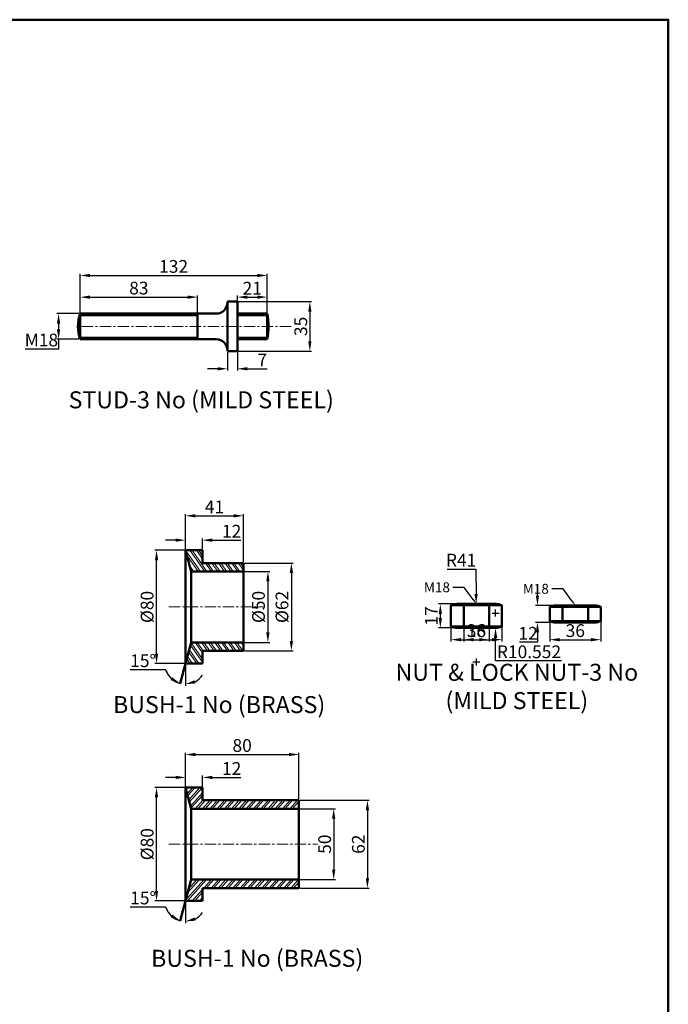
# Model space of a CAD drawing. Units: millimetres. Extents: x -98 to 907, y -783 to 313.
# Tile 3 of 3: x 449 to 907, y -383 to 313. Entities that reach past the tile are written whole.
import ezdxf
from ezdxf import colors
from ezdxf.entities.mleader import LeaderData, LeaderLine
from ezdxf.math import Vec2, Vec3

# ---------------------------------------------------------------- set-up
doc = ezdxf.new("R2010")
doc.units = ezdxf.units.MM
doc.header["$LTSCALE"] = 0.5
doc.linetypes.add('CENTER', pattern=[50.8, 31.75, -6.35, 6.35, -6.35])
for name, color, linetype, lineweight in [('M-CNTR', 1, 'CENTER', 18), ('M-DIMS', 2, 'Continuous', 25), ('M-HATC', 8, 'Continuous', 18), ('M-OUTL', 7, 'Continuous', 50), ('M-TEXT', 3, 'Continuous', 25)]:
    doc.layers.add(name, color=color, linetype=linetype, lineweight=lineweight)
doc.styles.get("Standard").update_dxf_attribs({"font": 'arial.ttf'})
doc.dimstyles.new('ISO-25', dxfattribs={"dimtxt": 9, "dimasz": 7, "dimexe": 1.25, "dimexo": 0.625, "dimtad": 1, "dimtoh": 1, "dimtxsty": 'Standard', "dimcen": 2.5, "dimadec": 0, "dimazin": 0, "dimtfac": 1, "dimtofl": 0, "dimtmove": 0, "dimatfit": 3, "dimfxl": 1, "dimarcsym": 0})

# ---------------------------------------------------------------- blocks, each defined once
blk = doc.blocks.new('*D15')
at = {"layer": 'Defpoints', "color": 0, "ltscale": 0.5, "transparency": 16777216}
for p in [(623.45, 132.18), (491.45, 105.21), (623.45, 105.21)]:
    blk.add_point(p, dxfattribs=at)
at = {"layer": 'M-DIMS', "color": 0, "lineweight": -2, "ltscale": 0.5, "transparency": 16777216}
for p, q in [((491.45, 105.84), (491.45, 133.43)), ((498.45, 132.18), (616.45, 132.18)), ((623.45, 105.84), (623.45, 133.43))]:
    blk.add_line(p, q, dxfattribs=at)
at = {"layer": 'M-DIMS', "color": 0, "ltscale": 0.5, "transparency": 16777216}
for points in [[(498.45, 133.35), (498.45, 131.02), (491.45, 132.18)], [(616.45, 133.35), (616.45, 131.02), (623.45, 132.18)]]:
    blk.add_solid(points, dxfattribs=at)
at = {"layer": 'M-DIMS', "color": 0, "ltscale": 0.5, "transparency": 16777216, "insert": (557.45, 137.41), "char_height": 9, "attachment_point": 5}
blk.add_mtext('132', dxfattribs=at)
blk = doc.blocks.new('*D16')
at = {"layer": 'Defpoints', "color": 0, "ltscale": 0.5, "transparency": 16777216}
for p in [(491.45, 111.42), (574.45, 116.88), (574.45, 104.21)]:
    blk.add_point(p, dxfattribs=at)
at = {"layer": 'M-DIMS', "color": 0, "lineweight": -2, "ltscale": 0.5, "transparency": 16777216}
for p, q in [((491.45, 112.04), (491.45, 118.13)), ((498.45, 116.88), (567.45, 116.88)), ((574.45, 104.84), (574.45, 118.13))]:
    blk.add_line(p, q, dxfattribs=at)
at = {"layer": 'M-DIMS', "color": 0, "ltscale": 0.5, "transparency": 16777216}
for points in [[(498.45, 118.04), (498.45, 115.71), (491.45, 116.88)], [(567.45, 118.04), (567.45, 115.71), (574.45, 116.88)]]:
    blk.add_solid(points, dxfattribs=at)
at = {"layer": 'M-DIMS', "color": 0, "ltscale": 0.5, "transparency": 16777216, "insert": (532.95, 122.1), "char_height": 9, "attachment_point": 5}
blk.add_mtext('83', dxfattribs=at)
blk = doc.blocks.new('*D17')
at = {"layer": 'Defpoints', "color": 0, "ltscale": 0.5, "transparency": 16777216}
for p in [(491.45, 105.21), (476.29, 87.21), (491.45, 87.21)]:
    blk.add_point(p, dxfattribs=at)
at = {"layer": 'M-DIMS', "color": 0, "lineweight": -2, "ltscale": 0.5, "transparency": 16777216}
for p, q in [((490.83, 105.21), (475.04, 105.21)), ((476.29, 98.21), (476.29, 94.21)), ((490.83, 87.21), (475.04, 87.21)), ((476.29, 87.21), (476.29, 80.21)), ((476.29, 80.21), (452.69, 80.21))]:
    blk.add_line(p, q, dxfattribs=at)
at = {"layer": 'M-DIMS', "color": 0, "ltscale": 0.5, "transparency": 16777216}
for points in [[(475.13, 98.21), (477.46, 98.21), (476.29, 105.21)], [(475.13, 94.21), (477.46, 94.21), (476.29, 87.21)]]:
    blk.add_solid(points, dxfattribs=at)
at = {"layer": 'M-DIMS', "color": 0, "ltscale": 0.5, "transparency": 16777216, "insert": (464.18, 85.43), "char_height": 9, "attachment_point": 5}
blk.add_mtext('M18', dxfattribs=at)
blk = doc.blocks.new('*D18')
at = {"layer": 'Defpoints', "color": 0, "ltscale": 0.5, "transparency": 16777216}
for p in [(595.45, 78.71), (602.45, 78.71), (602.45, 66.27)]:
    blk.add_point(p, dxfattribs=at)
at = {"layer": 'M-DIMS', "color": 0, "lineweight": -2, "ltscale": 0.5, "transparency": 16777216}
for p, q in [((595.45, 78.09), (595.45, 65.02)), ((602.45, 78.09), (602.45, 65.02)), ((588.45, 66.27), (581.45, 66.27)), ((609.45, 66.27), (623.53, 66.27))]:
    blk.add_line(p, q, dxfattribs=at)
at = {"layer": 'M-DIMS', "color": 0, "ltscale": 0.5, "transparency": 16777216}
for points in [[(588.45, 67.43), (588.45, 65.1), (595.45, 66.27)], [(609.45, 67.43), (609.45, 65.1), (602.45, 66.27)]]:
    blk.add_solid(points, dxfattribs=at)
at = {"layer": 'M-DIMS', "color": 0, "ltscale": 0.5, "transparency": 16777216, "insert": (619.99, 71.39), "char_height": 9, "attachment_point": 5}
blk.add_mtext('7', dxfattribs=at)
blk = doc.blocks.new('*D19')
at = {"layer": 'Defpoints', "color": 0, "ltscale": 0.5, "transparency": 16777216}
for p in [(602.45, 113.71), (623.45, 116.88), (623.45, 113.71)]:
    blk.add_point(p, dxfattribs=at)
at = {"layer": 'M-DIMS', "color": 0, "lineweight": -2, "ltscale": 0.5, "transparency": 16777216}
for p, q in [((602.45, 114.34), (602.45, 118.13)), ((609.45, 116.88), (616.45, 116.88)), ((623.45, 114.34), (623.45, 118.13))]:
    blk.add_line(p, q, dxfattribs=at)
at = {"layer": 'M-DIMS', "color": 0, "ltscale": 0.5, "transparency": 16777216}
for points in [[(609.45, 118.04), (609.45, 115.71), (602.45, 116.88)], [(616.45, 118.04), (616.45, 115.71), (623.45, 116.88)]]:
    blk.add_solid(points, dxfattribs=at)
at = {"layer": 'M-DIMS', "color": 0, "ltscale": 0.5, "transparency": 16777216, "insert": (612.95, 122.02), "char_height": 9, "attachment_point": 5}
blk.add_mtext('21', dxfattribs=at)
blk = doc.blocks.new('*D20')
at = {"layer": 'Defpoints', "color": 0, "ltscale": 0.5, "transparency": 16777216}
for p in [(602.45, 113.71), (602.45, 78.71), (653.62, 78.71)]:
    blk.add_point(p, dxfattribs=at)
at = {"layer": 'M-DIMS', "color": 0, "lineweight": -2, "ltscale": 0.5, "transparency": 16777216}
for p, q in [((603.08, 113.71), (654.87, 113.71)), ((653.62, 106.71), (653.62, 85.71)), ((603.08, 78.71), (654.87, 78.71))]:
    blk.add_line(p, q, dxfattribs=at)
at = {"layer": 'M-DIMS', "color": 0, "ltscale": 0.5, "transparency": 16777216}
for points in [[(652.45, 106.71), (654.78, 106.71), (653.62, 113.71)], [(652.45, 85.71), (654.78, 85.71), (653.62, 78.71)]]:
    blk.add_solid(points, dxfattribs=at)
at = {"layer": 'M-DIMS', "color": 0, "ltscale": 0.5, "transparency": 16777216, "insert": (648.39, 96.21), "char_height": 9, "attachment_point": 5, "rotation": 90}
blk.add_mtext('35', dxfattribs=at)
blk = doc.blocks.new('*D21')
at = {"layer": 'Defpoints', "color": 0, "ltscale": 0.5, "transparency": 16777216}
for p in [(577.83, -54.77), (565.83, -61.94), (577.83, -61.94)]:
    blk.add_point(p, dxfattribs=at)
at = {"layer": 'M-DIMS', "color": 0, "lineweight": -2, "ltscale": 0.5, "transparency": 16777216}
for p, q in [((558.83, -54.77), (551.83, -54.77)), ((565.83, -61.31), (565.83, -53.52)), ((577.83, -61.31), (577.83, -53.52)), ((584.83, -54.77), (605.03, -54.77))]:
    blk.add_line(p, q, dxfattribs=at)
at = {"layer": 'M-DIMS', "color": 0, "ltscale": 0.5, "transparency": 16777216}
for points in [[(558.83, -53.6), (558.83, -55.94), (565.83, -54.77)], [(584.83, -53.6), (584.83, -55.94), (577.83, -54.77)]]:
    blk.add_solid(points, dxfattribs=at)
at = {"layer": 'M-DIMS', "color": 0, "ltscale": 0.5, "transparency": 16777216, "insert": (598.43, -49.63), "char_height": 9, "attachment_point": 5}
blk.add_mtext('12', dxfattribs=at)
blk = doc.blocks.new('*D22')
at = {"layer": 'Defpoints', "color": 0, "ltscale": 0.5, "transparency": 16777216}
for p in [(606.83, -37.58), (565.83, -61.94), (606.83, -70.94)]:
    blk.add_point(p, dxfattribs=at)
at = {"layer": 'M-DIMS', "color": 0, "lineweight": -2, "ltscale": 0.5, "transparency": 16777216}
for p, q in [((565.83, -61.31), (565.83, -36.33)), ((572.83, -37.58), (599.83, -37.58)), ((606.83, -70.31), (606.83, -36.33))]:
    blk.add_line(p, q, dxfattribs=at)
at = {"layer": 'M-DIMS', "color": 0, "ltscale": 0.5, "transparency": 16777216}
for points in [[(572.83, -36.41), (572.83, -38.74), (565.83, -37.58)], [(599.83, -36.41), (599.83, -38.74), (606.83, -37.58)]]:
    blk.add_solid(points, dxfattribs=at)
at = {"layer": 'M-DIMS', "color": 0, "ltscale": 0.5, "transparency": 16777216, "insert": (586.33, -32.43), "char_height": 9, "attachment_point": 5}
blk.add_mtext('41', dxfattribs=at)
blk = doc.blocks.new('*D23')
at = {"layer": 'Defpoints', "color": 0, "ltscale": 0.5, "transparency": 16777216}
for p in [(606.83, -70.94), (606.83, -132.94), (640.59, -132.94)]:
    blk.add_point(p, dxfattribs=at)
at = {"layer": 'M-DIMS', "color": 0, "lineweight": -2, "ltscale": 0.5, "transparency": 16777216}
for p, q in [((607.45, -70.94), (641.84, -70.94)), ((640.59, -77.94), (640.59, -125.94)), ((607.45, -132.94), (641.84, -132.94))]:
    blk.add_line(p, q, dxfattribs=at)
at = {"layer": 'M-DIMS', "color": 0, "ltscale": 0.5, "transparency": 16777216}
for points in [[(639.42, -77.94), (641.76, -77.94), (640.59, -70.94)], [(639.42, -125.94), (641.76, -125.94), (640.59, -132.94)]]:
    blk.add_solid(points, dxfattribs=at)
at = {"layer": 'M-DIMS', "color": 0, "ltscale": 0.5, "transparency": 16777216, "insert": (635.12, -101.94), "char_height": 9, "attachment_point": 5, "rotation": 90}
blk.add_mtext('%%C62', dxfattribs=at)
blk = doc.blocks.new('*D24')
at = {"layer": 'Defpoints', "color": 0, "ltscale": 0.5, "transparency": 16777216}
for p in [(606.83, -76.94), (606.83, -126.94), (624.02, -126.94)]:
    blk.add_point(p, dxfattribs=at)
at = {"layer": 'M-DIMS', "color": 0, "lineweight": -2, "ltscale": 0.5, "transparency": 16777216}
for p, q in [((607.45, -76.94), (625.27, -76.94)), ((624.02, -83.94), (624.02, -119.94)), ((607.45, -126.94), (625.27, -126.94))]:
    blk.add_line(p, q, dxfattribs=at)
at = {"layer": 'M-DIMS', "color": 0, "ltscale": 0.5, "transparency": 16777216}
for points in [[(622.85, -83.94), (625.18, -83.94), (624.02, -76.94)], [(622.85, -119.94), (625.18, -119.94), (624.02, -126.94)]]:
    blk.add_solid(points, dxfattribs=at)
at = {"layer": 'M-DIMS', "color": 0, "ltscale": 0.5, "transparency": 16777216, "insert": (618.54, -101.94), "char_height": 9, "attachment_point": 5, "rotation": 90}
blk.add_mtext('%%C50', dxfattribs=at)
blk = doc.blocks.new('*D25')
at = {"layer": 'Defpoints', "color": 0, "ltscale": 0.5, "transparency": 16777216}
for p in [(545.42, -61.94), (565.83, -61.94), (565.83, -141.94)]:
    blk.add_point(p, dxfattribs=at)
at = {"layer": 'M-DIMS', "color": 0, "lineweight": -2, "ltscale": 0.5, "transparency": 16777216}
for p, q in [((565.2, -61.94), (544.17, -61.94)), ((545.42, -134.94), (545.42, -68.94)), ((565.2, -141.94), (544.17, -141.94))]:
    blk.add_line(p, q, dxfattribs=at)
at = {"layer": 'M-DIMS', "color": 0, "ltscale": 0.5, "transparency": 16777216}
for points in [[(544.26, -68.94), (546.59, -68.94), (545.42, -61.94)], [(544.26, -134.94), (546.59, -134.94), (545.42, -141.94)]]:
    blk.add_solid(points, dxfattribs=at)
at = {"layer": 'M-DIMS', "color": 0, "ltscale": 0.5, "transparency": 16777216, "insert": (539.95, -101.94), "char_height": 9, "attachment_point": 5, "rotation": 90}
blk.add_mtext('%%C80', dxfattribs=at)
blk = doc.blocks.new('*D26')
at = {"layer": 'Defpoints', "color": 0, "ltscale": 0.5, "transparency": 16777216}
for p in [(565.83, -101.94), (569.85, -126.94), (565.83, -141.94), (562.06, -156), (564.56, -156.44)]:
    blk.add_point(p, dxfattribs=at)
at = {"layer": 'M-DIMS', "color": 0, "lineweight": -2, "ltscale": 0.5, "transparency": 16777216}
for p, q in [((565.83, -142.56), (565.83, -157.74)), ((551.95, -146.31), (526.89, -146.31))]:
    blk.add_line(p, q, dxfattribs=at)
for start, end in [(197.5003, 255), (199.33739, 227.16869), (297.83131, 325.66261)]:
    blk.add_arc((565.83, -141.94), 14.55, start, end, dxfattribs=at)
at = {"layer": 'M-DIMS', "color": 0, "ltscale": 0.5, "transparency": 16777216}
for points in [[(556.5, -151.59), (555.37, -153.63), (562.06, -156)], [(572.9, -155.94), (572.34, -153.68), (565.83, -156.49)]]:
    blk.add_solid(points, dxfattribs=at)
at = {"layer": 'M-DIMS', "color": 0, "ltscale": 0.5, "transparency": 16777216, "insert": (535.92, -141.09), "char_height": 9, "attachment_point": 5}
blk.add_mtext('15°', dxfattribs=at)
blk = doc.blocks.new('*D29')
at = {"layer": 'Defpoints', "color": 0, "ltscale": 0.5, "transparency": 16777216}
for p in [(577.83, -222.33), (565.83, -229.5), (577.83, -229.5)]:
    blk.add_point(p, dxfattribs=at)
at = {"layer": 'M-DIMS', "color": 0, "lineweight": -2, "ltscale": 0.5, "transparency": 16777216}
for p, q in [((558.83, -222.33), (551.83, -222.33)), ((565.83, -228.88), (565.83, -221.08)), ((577.83, -228.88), (577.83, -221.08)), ((584.83, -222.33), (605.03, -222.33))]:
    blk.add_line(p, q, dxfattribs=at)
at = {"layer": 'M-DIMS', "color": 0, "ltscale": 0.5, "transparency": 16777216}
for points in [[(558.83, -221.17), (558.83, -223.5), (565.83, -222.33)], [(584.83, -221.17), (584.83, -223.5), (577.83, -222.33)]]:
    blk.add_solid(points, dxfattribs=at)
at = {"layer": 'M-DIMS', "color": 0, "ltscale": 0.5, "transparency": 16777216, "insert": (598.43, -217.19), "char_height": 9, "attachment_point": 5}
blk.add_mtext('12', dxfattribs=at)
blk = doc.blocks.new('*D27')
at = {"layer": 'Defpoints', "color": 0, "ltscale": 0.5, "transparency": 16777216}
for p in [(545.42, -229.5), (565.83, -229.5), (565.83, -309.5)]:
    blk.add_point(p, dxfattribs=at)
at = {"layer": 'M-DIMS', "color": 0, "lineweight": -2, "ltscale": 0.5, "transparency": 16777216}
for p, q in [((565.2, -229.5), (544.17, -229.5)), ((545.42, -302.5), (545.42, -236.5)), ((565.2, -309.5), (544.17, -309.5))]:
    blk.add_line(p, q, dxfattribs=at)
at = {"layer": 'M-DIMS', "color": 0, "ltscale": 0.5, "transparency": 16777216}
for points in [[(544.26, -236.5), (546.59, -236.5), (545.42, -229.5)], [(544.26, -302.5), (546.59, -302.5), (545.42, -309.5)]]:
    blk.add_solid(points, dxfattribs=at)
at = {"layer": 'M-DIMS', "color": 0, "ltscale": 0.5, "transparency": 16777216, "insert": (539.95, -269.5), "char_height": 9, "attachment_point": 5, "rotation": 90}
blk.add_mtext('%%C80', dxfattribs=at)
blk = doc.blocks.new('*D28')
at = {"layer": 'Defpoints', "color": 0, "ltscale": 0.5, "transparency": 16777216}
for p in [(565.83, -269.5), (569.85, -294.5), (565.83, -309.5), (562.06, -323.56), (564.56, -324)]:
    blk.add_point(p, dxfattribs=at)
at = {"layer": 'M-DIMS', "color": 0, "lineweight": -2, "ltscale": 0.5, "transparency": 16777216}
for p, q in [((565.83, -310.13), (565.83, -325.31)), ((551.95, -313.88), (526.89, -313.88))]:
    blk.add_line(p, q, dxfattribs=at)
for start, end in [(197.5003, 255), (199.33739, 227.16869), (297.83131, 325.66261)]:
    blk.add_arc((565.83, -309.5), 14.55, start, end, dxfattribs=at)
at = {"layer": 'M-DIMS', "color": 0, "ltscale": 0.5, "transparency": 16777216}
for points in [[(556.5, -319.15), (555.37, -321.2), (562.06, -323.56)], [(572.9, -323.51), (572.34, -321.24), (565.83, -324.06)]]:
    blk.add_solid(points, dxfattribs=at)
at = {"layer": 'M-DIMS', "color": 0, "ltscale": 0.5, "transparency": 16777216, "insert": (535.92, -308.66), "char_height": 9, "attachment_point": 5}
blk.add_mtext('15°', dxfattribs=at)
blk = doc.blocks.new('*D30')
at = {"layer": 'Defpoints', "color": 0, "ltscale": 0.5, "transparency": 16777216}
for p in [(645.83, -244.5), (645.83, -294.5), (670.45, -294.5)]:
    blk.add_point(p, dxfattribs=at)
at = {"layer": 'M-DIMS', "color": 0, "lineweight": -2, "ltscale": 0.5, "transparency": 16777216}
for p, q in [((646.45, -244.5), (671.7, -244.5)), ((670.45, -251.5), (670.45, -287.5)), ((646.45, -294.5), (671.7, -294.5))]:
    blk.add_line(p, q, dxfattribs=at)
at = {"layer": 'M-DIMS', "color": 0, "ltscale": 0.5, "transparency": 16777216}
for points in [[(669.29, -251.5), (671.62, -251.5), (670.45, -244.5)], [(669.29, -287.5), (671.62, -287.5), (670.45, -294.5)]]:
    blk.add_solid(points, dxfattribs=at)
at = {"layer": 'M-DIMS', "color": 0, "ltscale": 0.5, "transparency": 16777216, "insert": (665.23, -269.5), "char_height": 9, "attachment_point": 5, "rotation": 90}
blk.add_mtext('50', dxfattribs=at)
blk = doc.blocks.new('*D31')
at = {"layer": 'Defpoints', "color": 0, "ltscale": 0.5, "transparency": 16777216}
for p in [(645.83, -238.5), (645.83, -300.5), (694.26, -300.5)]:
    blk.add_point(p, dxfattribs=at)
at = {"layer": 'M-DIMS', "color": 0, "lineweight": -2, "ltscale": 0.5, "transparency": 16777216}
for p, q in [((646.45, -238.5), (695.51, -238.5)), ((694.26, -245.5), (694.26, -293.5)), ((646.45, -300.5), (695.51, -300.5))]:
    blk.add_line(p, q, dxfattribs=at)
at = {"layer": 'M-DIMS', "color": 0, "ltscale": 0.5, "transparency": 16777216}
for points in [[(693.09, -245.5), (695.42, -245.5), (694.26, -238.5)], [(693.09, -293.5), (695.42, -293.5), (694.26, -300.5)]]:
    blk.add_solid(points, dxfattribs=at)
at = {"layer": 'M-DIMS', "color": 0, "ltscale": 0.5, "transparency": 16777216, "insert": (689.04, -269.5), "char_height": 9, "attachment_point": 5, "rotation": 90}
blk.add_mtext('62', dxfattribs=at)
blk = doc.blocks.new('*D32')
at = {"layer": 'Defpoints', "color": 0, "ltscale": 0.5, "transparency": 16777216}
for p in [(645.83, -206.17), (565.83, -229.5), (645.83, -238.5)]:
    blk.add_point(p, dxfattribs=at)
at = {"layer": 'M-DIMS', "color": 0, "lineweight": -2, "ltscale": 0.5, "transparency": 16777216}
for p, q in [((565.83, -228.88), (565.83, -204.92)), ((572.83, -206.17), (638.83, -206.17)), ((645.83, -237.88), (645.83, -204.92))]:
    blk.add_line(p, q, dxfattribs=at)
at = {"layer": 'M-DIMS', "color": 0, "ltscale": 0.5, "transparency": 16777216}
for points in [[(572.83, -205.01), (572.83, -207.34), (565.83, -206.17)], [(638.83, -205.01), (638.83, -207.34), (645.83, -206.17)]]:
    blk.add_solid(points, dxfattribs=at)
at = {"layer": 'M-DIMS', "color": 0, "ltscale": 0.5, "transparency": 16777216, "insert": (605.83, -200.95), "char_height": 9, "attachment_point": 5}
blk.add_mtext('80', dxfattribs=at)
blk = doc.blocks.new('*D33')
at = {"layer": 'Defpoints', "color": 0, "ltscale": 0.5, "transparency": 16777216}
for p in [(762.2, -99.8), (745.71, -116.8), (762.2, -116.8)]:
    blk.add_point(p, dxfattribs=at)
at = {"layer": 'M-DIMS', "color": 0, "lineweight": -2, "ltscale": 0.5, "transparency": 16777216}
for p, q in [((761.57, -99.8), (744.46, -99.8)), ((745.71, -106.8), (745.71, -109.8)), ((761.57, -116.8), (744.46, -116.8))]:
    blk.add_line(p, q, dxfattribs=at)
at = {"layer": 'M-DIMS', "color": 0, "ltscale": 0.5, "transparency": 16777216}
for points in [[(744.54, -106.8), (746.87, -106.8), (745.71, -99.8)], [(744.54, -109.8), (746.87, -109.8), (745.71, -116.8)]]:
    blk.add_solid(points, dxfattribs=at)
at = {"layer": 'M-DIMS', "color": 0, "ltscale": 0.5, "transparency": 16777216, "insert": (740.56, -108.3), "char_height": 9, "attachment_point": 5, "rotation": 90}
blk.add_mtext('17', dxfattribs=at)
blk = doc.blocks.new('*D34')
at = {"layer": 'Defpoints', "color": 0, "ltscale": 0.5, "transparency": 16777216}
for p in [(831.97, -100.88), (814.24, -112.88), (831.97, -112.88)]:
    blk.add_point(p, dxfattribs=at)
at = {"layer": 'M-DIMS', "color": 0, "lineweight": -2, "ltscale": 0.5, "transparency": 16777216}
for p, q in [((814.24, -93.88), (814.24, -86.88)), ((831.34, -100.88), (812.99, -100.88)), ((831.34, -112.88), (812.99, -112.88)), ((814.24, -119.88), (814.24, -126.88)), ((814.24, -126.88), (801.67, -126.88))]:
    blk.add_line(p, q, dxfattribs=at)
at = {"layer": 'M-DIMS', "color": 0, "ltscale": 0.5, "transparency": 16777216}
for points in [[(813.08, -93.88), (815.41, -93.88), (814.24, -100.88)], [(813.08, -119.88), (815.41, -119.88), (814.24, -112.88)]]:
    blk.add_solid(points, dxfattribs=at)
at = {"layer": 'M-DIMS', "color": 0, "ltscale": 0.5, "transparency": 16777216, "insert": (807.64, -121.73), "char_height": 9, "attachment_point": 5}
blk.add_mtext('12', dxfattribs=at)
blk = doc.blocks.new('NUT-HEX')
at = {"ltscale": 0.5}
for p, q in [((0, 16.01), (36, 16.01)), ((0, 8.51), (0, 16.01)), ((9, 8.51), (9, 17.01)), ((27, 17.01), (27, 8.51)), ((36, 16.01), (36, 8.51)), ((0, 1.01), (0, 8.51)), ((9, 1.01), (9, 8.51)), ((27, 8.51), (27, 1.01)), ((36, 8.51), (36, 1.01)), ((36, 1.01), (0, 1.01))]:
    blk.add_line(p, q, dxfattribs=at)
for centre, radius, start, end in [((4.5, 6.44), 10.57, 64.81518, 115.18482), ((18, -23.99), 41, 77.31962, 102.68038), ((31.5, 6.46), 10.55, 64.75651, 115.24349), ((4.5, 10.58), 10.57, 244.81518, 295.18482), ((18, 41.01), 41, 257.31962, 282.68038), ((31.5, 10.55), 10.55, 244.75651, 295.24349)]:
    blk.add_arc(centre, radius, start, end, dxfattribs=at)
blk = doc.blocks.new('STUD')
at = {"ltscale": 0.5}
for p, q in [((595.45, 113.71), (595.45, 78.71)), ((602.45, 113.71), (595.45, 113.71)), ((602.45, 78.71), (602.45, 113.71)), ((491.45, 105.21), (587.45, 105.21)), ((491.45, 87.21), (491.45, 105.21)), ((587.45, 87.21), (491.45, 87.21)), ((595.45, 78.71), (602.45, 78.71))]:
    blk.add_line(p, q, dxfattribs=at)
for centre, radius, start, end in [((587.45, 113.21), 8, 270, 0), ((517.57, 96.21), 27.63, 160.98867, 199.01133), ((587.45, 79.21), 8, 0, 90)]:
    blk.add_arc(centre, radius, start, end, dxfattribs=at)
blk = doc.blocks.new('*D38')
at = {"layer": 'Defpoints', "color": 0, "ltscale": 0.5, "transparency": 16777216}
for p in [(753.2, -100.8), (789.2, -100.8), (789.2, -125.05)]:
    blk.add_point(p, dxfattribs=at)
at = {"layer": 'M-DIMS', "color": 0, "lineweight": -2, "ltscale": 0.5, "transparency": 16777216}
for p, q in [((753.2, -101.42), (753.2, -126.3)), ((789.2, -101.42), (789.2, -126.3)), ((760.2, -125.05), (782.2, -125.05))]:
    blk.add_line(p, q, dxfattribs=at)
at = {"layer": 'M-DIMS', "color": 0, "ltscale": 0.5, "transparency": 16777216}
for points in [[(760.2, -123.89), (760.2, -126.22), (753.2, -125.05)], [(782.2, -123.89), (782.2, -126.22), (789.2, -125.05)]]:
    blk.add_solid(points, dxfattribs=at)
at = {"layer": 'M-DIMS', "color": 0, "ltscale": 0.5, "transparency": 16777216, "insert": (771.2, -119.83), "char_height": 9, "attachment_point": 5}
blk.add_mtext('36', dxfattribs=at)
blk = doc.blocks.new('*D39')
at = {"layer": 'Defpoints', "color": 0, "ltscale": 0.5, "transparency": 16777216}
for p in [(762.2, -115.8), (780.2, -115.8), (780.2, -125.05)]:
    blk.add_point(p, dxfattribs=at)
at = {"layer": 'M-DIMS', "color": 0, "lineweight": -2, "ltscale": 0.5, "transparency": 16777216}
for p, q in [((762.2, -116.42), (762.2, -126.3)), ((780.2, -116.42), (780.2, -126.3)), ((769.2, -125.05), (773.2, -125.05))]:
    blk.add_line(p, q, dxfattribs=at)
at = {"layer": 'M-DIMS', "color": 0, "ltscale": 0.5, "transparency": 16777216}
for points in [[(769.2, -123.89), (769.2, -126.22), (762.2, -125.05)], [(773.2, -123.89), (773.2, -126.22), (780.2, -125.05)]]:
    blk.add_solid(points, dxfattribs=at)
at = {"layer": 'M-DIMS', "color": 0, "ltscale": 0.5, "transparency": 16777216, "insert": (771.2, -119.83), "char_height": 9, "attachment_point": 5}
blk.add_mtext('18', dxfattribs=at)
blk = doc.blocks.new('*D40')
at = {"layer": 'Defpoints', "color": 0, "ltscale": 0.5, "transparency": 16777216}
for p in [(822.97, -101.88), (858.97, -101.88), (858.97, -125.05)]:
    blk.add_point(p, dxfattribs=at)
at = {"layer": 'M-DIMS', "color": 0, "lineweight": -2, "ltscale": 0.5, "transparency": 16777216}
for p, q in [((822.97, -102.5), (822.97, -126.3)), ((858.97, -102.5), (858.97, -126.3)), ((829.97, -125.05), (851.97, -125.05))]:
    blk.add_line(p, q, dxfattribs=at)
at = {"layer": 'M-DIMS', "color": 0, "ltscale": 0.5, "transparency": 16777216}
for points in [[(829.97, -123.89), (829.97, -126.22), (822.97, -125.05)], [(851.97, -123.89), (851.97, -126.22), (858.97, -125.05)]]:
    blk.add_solid(points, dxfattribs=at)
at = {"layer": 'M-DIMS', "color": 0, "ltscale": 0.5, "transparency": 16777216, "insert": (840.97, -119.83), "char_height": 9, "attachment_point": 5}
blk.add_mtext('36', dxfattribs=at)
blk = doc.blocks.new('*D52')
at = {"layer": 'Defpoints', "color": 0, "ltscale": 0.5, "transparency": 16777216}
for p in [(771, -99.8), (771.2, -140.8)]:
    blk.add_point(p, dxfattribs=at)
at = {"layer": 'M-DIMS', "color": 0, "lineweight": -2, "ltscale": 0.5, "transparency": 16777216}
for p, q in [((750.49, -75.2), (770.88, -75.2)), ((770.88, -75.2), (770.97, -92.8)), ((771.2, -143.3), (771.2, -138.3)), ((768.7, -140.8), (773.7, -140.8))]:
    blk.add_line(p, q, dxfattribs=at)
at = {"layer": 'M-DIMS', "color": 0, "ltscale": 0.5, "transparency": 16777216}
blk.add_solid([(772.13, -92.79), (769.8, -92.8), (771, -99.8)], dxfattribs=at)
at = {"layer": 'M-DIMS', "color": 0, "ltscale": 0.5, "transparency": 16777216, "insert": (760.37, -70.05), "char_height": 9, "attachment_point": 5}
blk.add_mtext('R41', dxfattribs=at)
blk = doc.blocks.new('*D53')
at = {"layer": 'Defpoints', "color": 0, "ltscale": 0.5, "transparency": 16777216}
for p in [(784.7, -106.25), (784.7, -116.8)]:
    blk.add_point(p, dxfattribs=at)
at = {"layer": 'M-DIMS', "color": 0, "lineweight": -2, "ltscale": 0.5, "transparency": 16777216}
for p, q in [((784.7, -108.75), (784.7, -103.75)), ((782.2, -106.25), (787.2, -106.25)), ((784.7, -139.99), (784.7, -123.8)), ((831.21, -139.99), (784.7, -139.99))]:
    blk.add_line(p, q, dxfattribs=at)
at = {"layer": 'M-DIMS', "color": 0, "ltscale": 0.5, "transparency": 16777216}
blk.add_solid([(785.87, -123.8), (783.53, -123.8), (784.7, -116.8)], dxfattribs=at)
at = {"layer": 'M-DIMS', "color": 0, "ltscale": 0.5, "transparency": 16777216, "insert": (808.27, -134.77), "char_height": 9, "attachment_point": 5}
blk.add_mtext('R10.552', dxfattribs=at)

msp = doc.modelspace()

# ---------------------------------------------------------------- hatches: boundary and pattern name
at = {"layer": 'M-HATC', "ltscale": 0.5}
h = msp.add_hatch(dxfattribs=at)
h.set_pattern_fill('ANSI32', color=256, scale=0.4, angle=80)
h.paths.add_polyline_path([(606.8289, -70.9377), (577.8289, -70.9377), (577.8289, -61.9377), (565.8289, -61.9377), (569.8482, -76.9377), (606.8289, -76.9377)])
h.paths.add_polyline_path([(577.8289, -132.9377), (606.8289, -132.9377), (606.8289, -126.9377), (569.8482, -126.9377), (565.8289, -141.9377), (577.8289, -141.9377)])
h = msp.add_hatch(dxfattribs=at)
h.set_pattern_fill('ANSI32', color=256, scale=0.4, angle=183)
h.paths.add_polyline_path([(645.8289, -238.5028), (577.8289, -238.5028), (577.8289, -229.5028), (565.8289, -229.5028), (569.8482, -244.5028), (645.8289, -244.5028)])
h.paths.add_polyline_path([(645.8289, -294.5028), (569.8482, -294.5028), (565.8289, -309.5028), (577.8289, -309.5028), (577.8289, -300.5028), (645.8289, -300.5028)])

# ---------------------------------------------------------------- linework, layer by layer
at = {"layer": 'M-CNTR', "ltscale": 0.5}
for p, q in [((640.3985, 96.2123), (491.4507, 96.2123)), ((554.1108, -101.9377), (620.7669, -101.9377)), ((554.1108, -269.5028), (659.0179, -269.5028))]:
    msp.add_line(p, q, dxfattribs=at)
at = {"layer": 'M-OUTL', "ltscale": 0.5}
for p, q in [((574.4507, 87.2123), (574.4507, 105.2123)), ((602.4507, 105.2123), (623.4507, 105.2123)), ((623.4507, 87.2123), (623.4507, 105.2123)), ((491.4507, 104.2123), (574.4507, 104.2123)), ((602.4507, 104.2123), (623.4507, 104.2123)), ((574.4507, 88.2123), (491.4507, 88.2123)), ((623.4507, 88.2123), (602.4507, 88.2123)), ((623.4507, 87.2123), (602.4507, 87.2123)), ((565.8289, -61.9377), (565.8289, -101.9377)), ((577.8289, -61.9377), (565.8289, -61.9377)), ((569.8482, -76.9377), (565.8289, -61.9377)), ((577.8289, -70.9377), (577.8289, -61.9377)), ((606.8289, -70.9377), (577.8289, -70.9377)), ((606.8289, -101.9377), (606.8289, -70.9377)), ((606.8289, -76.9377), (569.8482, -76.9377)), ((569.8482, -76.9377), (569.8482, -126.9377)), ((565.8289, -141.9377), (565.8289, -101.9377)), ((606.8289, -101.9377), (606.8289, -132.9377)), ((757.3651, -99.7966), (785.1001, -99.7966)), ((827.1368, -100.8763), (854.8718, -100.8763)), ((757.3651, -116.7966), (785.1001, -116.7966)), ((827.1368, -112.8763), (854.8718, -112.8763)), ((569.8482, -126.9377), (562.0622, -155.9953)), ((606.8289, -126.9377), (569.8482, -126.9377)), ((606.8289, -132.9377), (577.8289, -132.9377)), ((577.8289, -132.9377), (577.8289, -141.9377)), ((577.8289, -141.9377), (565.8289, -141.9377)), ((565.8289, -229.5028), (565.8289, -269.5028)), ((577.8289, -229.5028), (565.8289, -229.5028)), ((569.8482, -244.5028), (565.8289, -229.5028)), ((577.8289, -238.5028), (577.8289, -229.5028)), ((645.8289, -238.5028), (577.8289, -238.5028)), ((645.8289, -238.5028), (645.8289, -300.5028)), ((645.8289, -244.5028), (569.8482, -244.5028)), ((569.8482, -244.5028), (569.8482, -294.5028)), ((565.8289, -309.5028), (565.8289, -269.5028)), ((569.8482, -294.5028), (562.0622, -323.5603)), ((645.8289, -294.5028), (569.8482, -294.5028)), ((645.8289, -300.5028), (577.8289, -300.5028)), ((577.8289, -300.5028), (577.8289, -309.5028)), ((577.8289, -309.5028), (565.8289, -309.5028))]:
    msp.add_line(p, q, dxfattribs=at)
msp.add_lwpolyline([(-98.0885, 312.8308), (906.5931, 312.8308), (906.5931, -783.1771), (-98.0885, -783.1771)], close=True, dxfattribs=at)
msp.add_lwpolyline([(822.9698, -101.8763, -0.22338737), (831.9698, -101.8763, -0.11111111), (849.9698, -101.8763, -0.22392501), (858.9698, -101.8763), (822.9698, -101.8763), (822.9698, -106.8763), (822.9698, -111.8763, 0.22338737), (831.9698, -111.8763, 0.11111111), (849.9698, -111.8763, 0.22392501), (858.9698, -111.8763), (822.9698, -111.8763)], format="xyb", dxfattribs=at)
for points in [[(831.9698, -111.8763), (831.9698, -106.8763), (831.9698, -100.8763)], [(849.9698, -100.8763), (849.9698, -106.8763), (849.9698, -111.8763)], [(858.9698, -101.8763), (858.9698, -106.8763), (858.9698, -111.8763)]]:
    msp.add_lwpolyline(points, dxfattribs=at)
msp.add_arc((581.6531, 96.2123), 42.7556, 347.848408, 12.151592, dxfattribs=at)

# ---------------------------------------------------------------- block references
at = {"layer": 'M-OUTL'}
for name, p in [('STUD', (0, 0)), ('NUT-HEX', (753.198, -116.804))]:
    msp.add_blockref(name, p, dxfattribs=at)

# ---------------------------------------------------------------- texts
at = {"layer": 'M-TEXT', "ltscale": 0.5, "char_height": 12, "attachment_point": 1}
for s, width, insert in [('\\pxqc;STUD-3 No (MILD STEEL)', 200.637042, (476.6356, 50.3513)), ('\\pxqc;NUT & LOCK NUT-3 No (MILD STEEL)', 181.185119, (709.1159, -142.0741)), ('\\pxqc;BUSH-1 No (BRASS)', 181.185119, (499.0219, -164.9112)), ('\\pxqc;BUSH-1 No (BRASS)', 181.185119, (525.864, -344.1029))]:
    msp.add_mtext_dynamic_manual_height_columns(s, width=width, gutter_width=12.5, heights=[0], dxfattribs=dict(at, insert=insert))

# ---------------------------------------------------------------- dimensions: what is measured, and where the dimension line sits
at = {"layer": 'M-DIMS', "ltscale": 0.5}
for base, p1, p2, override, picture, middle in [((623.4507, 132.1848), (491.4507, 105.2123), (623.4507, 105.2123), {"dimclrd": 0, "dimclre": 0, "dimclrt": 0}, '*D15', (557.4507, 137.408)), ((574.4507, 116.8754), (491.4507, 111.4172), (574.4507, 104.2123), {"dimclrd": 0, "dimclre": 0, "dimclrt": 0}, '*D16', (532.9507, 122.0986)), ((623.4507, 116.8754), (602.4507, 113.7123), (623.4507, 113.7123), {"dimclrd": 0, "dimclre": 0, "dimclrt": 0}, '*D19', (612.9507, 122.0188)), ((602.4507, 66.2671), (595.4507, 78.7123), (602.4507, 78.7123), {"dimclrd": 0, "dimclre": 0, "dimclrt": 0}, '*D18', (619.9888, 71.3921)), ((606.8289, -37.577), (565.8289, -61.9377), (606.8289, -70.9377), {"dimclrd": 0, "dimclre": 0, "dimclrt": 0}, '*D22', (586.3289, -32.4336)), ((577.8289, -54.7698), (565.8289, -61.9377), (577.8289, -61.9377), {"dimclrd": 0, "dimclre": 0, "dimclrt": 0}, '*D21', (598.4304, -49.6264)), ((789.1981, -125.0543), (753.1981, -100.7966), (789.1981, -100.7966), {"dimdec": 0, "dimlfac": 1, "dimrnd": 0, "dimzin": 0, "dimdsep": 46, "dimlunit": 2}, '*D38', (771.1981, -119.8311)), ((858.9698, -125.0543), (822.9698, -101.8763), (858.9698, -101.8763), {"dimdec": 0, "dimlfac": 1, "dimrnd": 0, "dimzin": 0, "dimdsep": 46, "dimlunit": 2}, '*D40', (840.9698, -119.8311)), ((780.1981, -125.0543), (762.1981, -115.7966), (780.1981, -115.7966), {"dimdec": 0, "dimlfac": 1, "dimrnd": 0, "dimzin": 0, "dimdsep": 46, "dimlunit": 2}, '*D39', (771.1981, -119.8341)), ((645.8289, -206.1722), (565.8289, -229.5028), (645.8289, -238.5028), {"dimclrd": 0, "dimclre": 0, "dimclrt": 0}, '*D32', (605.8289, -200.952)), ((577.8289, -222.3349), (565.8289, -229.5028), (577.8289, -229.5028), {"dimclrd": 0, "dimclre": 0, "dimclrt": 0}, '*D29', (598.4304, -217.1915))]:
    dim = msp.add_linear_dim(base=base, p1=p1, p2=p2, dimstyle='ISO-25', override=override, dxfattribs=at)
    dim.commit()
    dim.dimension.update_dxf_attribs({"geometry": picture, "text_midpoint": middle})
for base, p1, p2, picture, middle in [((653.6172, 78.7123), (602.4507, 113.7123), (602.4507, 78.7123), '*D20', (648.394, 96.2123)), ((814.2441, -112.8763), (831.9698, -100.8763), (831.9698, -112.8763), '*D34', (807.6427, -121.7329)), ((745.7083, -116.7966), (762.1981, -99.7966), (762.1981, -116.7966), '*D33', (740.5649, -108.2966)), ((694.2574, -300.5028), (645.8289, -238.5028), (645.8289, -300.5028), '*D31', (689.0372, -269.5028)), ((670.4533, -294.5028), (645.8289, -244.5028), (645.8289, -294.5028), '*D30', (665.2331, -269.5028))]:
    dim = msp.add_linear_dim(base=base, p1=p1, p2=p2, angle=90, dimstyle='ISO-25', override={"dimclrd": 0, "dimclre": 0, "dimclrt": 0}, dxfattribs=at)
    dim.commit()
    dim.dimension.update_dxf_attribs({"geometry": picture, "text_midpoint": middle})
for base, p1, p2, text, picture, middle in [((476.2917, 87.2123), (491.4507, 105.2123), (491.4507, 87.2123), 'M<>', '*D17', (464.1803, 85.4325)), ((545.4231, -61.9377), (565.8289, -141.9377), (565.8289, -61.9377), '%%C<>', '*D25', (539.9513, -101.9377)), ((640.5903, -132.9377), (606.8289, -70.9377), (606.8289, -132.9377), '%%C<>', '*D23', (635.1184, -101.9377)), ((624.0163, -126.9377), (606.8289, -76.9377), (606.8289, -126.9377), '%%C<>', '*D24', (618.5444, -101.9377)), ((545.4231, -229.5028), (565.8289, -309.5028), (565.8289, -229.5028), '%%C<>', '*D27', (539.9513, -269.5028))]:
    dim = msp.add_linear_dim(base=base, p1=p1, p2=p2, angle=90, text=text, dimstyle='ISO-25', override={"dimclrd": 0, "dimclre": 0, "dimclrt": 0}, dxfattribs=at)
    dim.commit()
    dim.dimension.update_dxf_attribs({"geometry": picture, "text_midpoint": middle})
dim = msp.add_radius_dim(center=(771.1981, -140.7966), mpoint=(771, -99.7971), dimstyle='ISO-25', override={"dimdec": 0, "dimlfac": 1, "dimrnd": 0, "dimzin": 0, "dimdsep": 46, "dimlunit": 2}, dxfattribs=at)
dim.commit()
dim.dimension.update_dxf_attribs({"geometry": '*D52', "text_midpoint": (760.3721, -75.1974), "dimtype": 164})
for base, line1, line2, picture, middle in [((564.5605, -156.4358), ((565.8289, -141.9377), (565.8289, -101.9377)), ((569.8482, -126.9377), (562.0622, -155.9953)), '*D26', (535.9196, -141.0939)), ((564.5605, -324.0008), ((565.8289, -309.5028), (565.8289, -269.5028)), ((569.8482, -294.5028), (562.0622, -323.5603)), '*D28', (535.9196, -308.659))]:
    dim = msp.add_angular_dim_2l(base=base, line1=line1, line2=line2, dimstyle='ISO-25', override={"dimclrd": 0, "dimclre": 0, "dimclrt": 0}, dxfattribs=at)
    dim.commit()
    dim.dimension.update_dxf_attribs({"geometry": picture, "text_midpoint": middle})
dim = msp.add_radius_dim(center=(784.6981, -106.2525), mpoint=(784.7, -116.8043), dimstyle='ISO-25', override={"dimdec": 3, "dimlfac": 1, "dimrnd": 0, "dimzin": 0, "dimdsep": 46, "dimlunit": 2}, dxfattribs=at)
dim.commit()
dim.dimension.update_dxf_attribs({"geometry": '*D53', "text_midpoint": (808.2712, -134.7745)})

# ---------------------------------------------------------------- leaders
at = {"layer": 'M-TEXT', "ltscale": 0.5}
ml = msp.add_multileader_mtext('Standard', dxfattribs=at)
ml.set_content('M18', color=256)
ml.set_leader_properties()
ml.build(insert=Vec2(0, 0))
ctx = ml.context
ctx.base_point, ctx.char_height, ctx.plane_origin = Vec3(732.6214, -88.095), 7, Vec3(771.1981, -99.7966)
ctx.text_align_type = 2
notes = []
notes.append((ctx, [(0, (1, 1, 0), (762.4891, -88.095), (-1, 0), 8, [(0, [(771.1981, -99.7966)], 0, [])])]))
ctx.mtext.insert, ctx.mtext.alignment, ctx.mtext.flow_direction = Vec3(752.4891, -84.5354), 3, 5
ml = msp.add_multileader_mtext('Standard', dxfattribs=at)
ml.set_content('M18', color=256)
ml.set_leader_properties()
ml.build(insert=Vec2(0, 0))
ctx = ml.context
ctx.base_point, ctx.char_height, ctx.plane_origin = Vec3(802.4277, -89.1747), 7, Vec3(841.0043, -100.8763)
ctx.text_align_type = 2
notes.append((ctx, [(0, (1, 1, 0), (832.2953, -89.1747), (-1, 0), 8, [(0, [(841.0043, -100.8763)], 0, [])])]))
ctx.mtext.insert, ctx.mtext.alignment, ctx.mtext.flow_direction = Vec3(822.2953, -85.615), 3, 5
for ctx, leaders in notes:
    for number, flags, end, landing, length, lines in leaders:
        leader = LeaderData()
        leader.index, (leader.has_last_leader_line, leader.has_dogleg_vector, leader.attachment_direction) = number, flags
        leader.last_leader_point, leader.dogleg_vector, leader.dogleg_length = Vec3(end), Vec3(landing), length
        for number, points, colour, breaks in lines:
            line = LeaderLine()
            line.index, line.vertices, line.color, line.breaks = number, Vec3.list(points), colors.encode_raw_color(colour), breaks
            leader.lines.append(line)
        ctx.leaders.append(leader)

doc.saveas('drawing.dxf')
